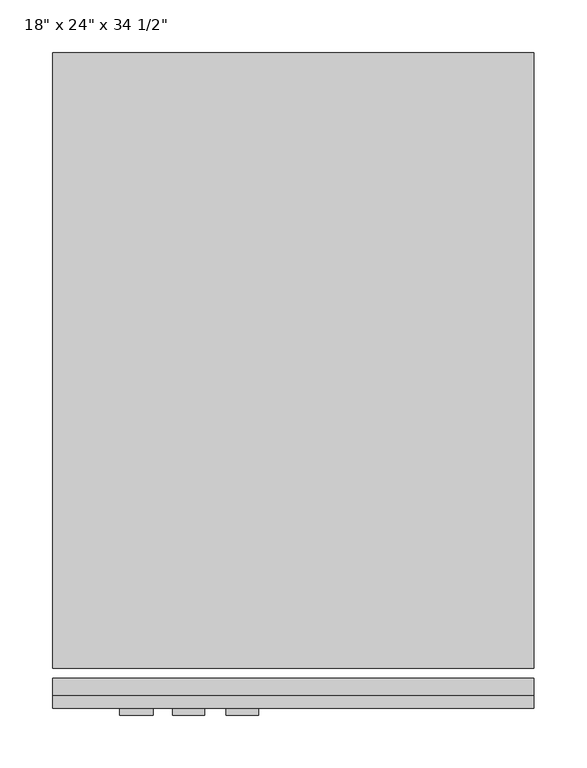
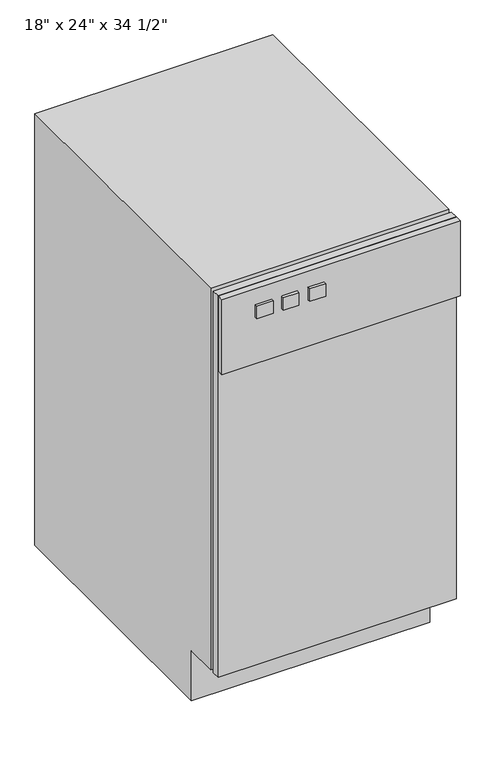
"""IFC4 building model written with IfcOpenShell, lengths in millimetres: proxy geometry."""

from ifc_helpers import new_model, si_unit, frame, origin, place, context, project, spatial, polyline, outline, extrude, source, transform, mapped, element, save


def proxy_7e1014cc(model_context):
    return source(origin(), model_context, "Body", "SweptSolid", [
        extrude(outline(polyline([(534.7174685, -38.3504352), (77.5174685, -38.3504352), (77.5174685, -22.4754352), (534.7174685, -22.4754352), (534.7174685, -38.3504352)])), frame((0.0, 0.0, 101.6), z_axis=(0.0, 0.0, 1.0), x_axis=(1.0, 0.0, 0.0)), (0.0, 0.0, 1.0), 774.7),
        extrude(outline(polyline([(534.7174685, -38.3504352), (534.7174685, -51.0504352), (77.5174685, -51.0504352), (77.5174685, -38.3504352), (534.7174685, -38.3504352)])), frame((0.0, 0.0, 723.9), z_axis=(0.0, 0.0, 1.0), x_axis=(1.0, 0.0, 0.0)), (0.0, 0.0, 1.0), 152.4),
        extrude(outline(polyline([(571.2495648, 0.0), (50.5495648, 0.0), (50.5495648, 101.6), (-12.9504352, 101.6), (-12.9504352, 876.3), (571.2495648, 876.3), (571.2495648, 0.0)])), frame((77.5174685, 0.0, 0.0), z_axis=(1.0, 0.0, 0.0), x_axis=(0.0, 1.0, 0.0)), (0.0, 0.0, 1.0), 457.2),
        extrude(outline(polyline([(172.7674685, -57.4004352), (141.0174685, -57.4004352), (141.0174685, -51.0504352), (172.7674685, -51.0504352), (172.7674685, -57.4004352)])), frame((0.0, 0.0, 818.6415009), z_axis=(0.0, 0.0, 1.0), x_axis=(1.0, 0.0, 0.0)), (0.0, 0.0, 1.0), 25.4),
        extrude(outline(polyline([(221.6847918, -57.4004352), (191.3389562, -57.4004352), (191.3389562, -51.0504352), (221.6847918, -51.0504352), (221.6847918, -57.4004352)])), frame((0.0, 0.0, 818.6415009), z_axis=(0.0, 0.0, 1.0), x_axis=(1.0, 0.0, 0.0)), (0.0, 0.0, 1.0), 25.4),
        extrude(outline(polyline([(272.969254, -57.4004352), (242.3199601, -57.4004352), (242.3199601, -51.0504352), (272.969254, -51.0504352), (272.969254, -57.4004352)])), frame((0.0, 0.0, 818.6415009), z_axis=(0.0, 0.0, 1.0), x_axis=(1.0, 0.0, 0.0)), (0.0, 0.0, 1.0), 25.4),
    ])


if __name__ == "__main__":
    model = new_model("IFC4")
    model_context = context("Model", 3, world=origin())
    ifc_project = project(units=[si_unit("LENGTHUNIT", "METRE", prefix="MILLI")], contexts=[model_context])
    site = spatial("IfcSite", under=ifc_project)
    building = spatial("IfcBuilding", under=site)
    placement = place(None, origin())
    proxy_shape = proxy_7e1014cc(model_context)
    element("IfcBuildingElementProxy", 1, Name="18\" x 24\" x 34 1/2\"", ObjectType="18\" x 24\" x 34 1/2\"", at=placement, inside=building, context=model_context, shape_type="MappedRepresentation", body=[
        mapped(proxy_shape, transform((0.0, 0.0, 0.0), x_axis=(1.0, 0.0, 0.0), y_axis=(0.0, 1.0, 0.0), z_axis=(0.0, 0.0, 1.0))),
    ])
    save(model, "model.ifc")

# Revit data of these elements
# Type "18\" x 24\" x 34 1/2\""
#   Label = "T"
#   Assembly Code = "E1090400"
#   Depth = 2' - 0"
#   Height = 2' - 10 1/2"
#   Width = 1' - 6"
#   Panel Face Material = Plastic, Opaque Black
#   Trach Compact. Material = Steel, Paint Finish, Ivory, Matte
#   Default Elevation = 0
# Element 1 (IfcBuildingElementProxy, "18\" x 24\" x 34 1/2\"")
#   Materials on its faces: "Steel, Paint Finish, Ivory, Matte", "Plastic, Opaque Black"
# Materials
#   "Plastic, Opaque Black": class "Plastic", colour RGB 0 0 0, transparency 0, Description = "Plastic, generic, opaque black", Cost = 0
#   "Steel, Paint Finish, Ivory, Matte": class "Metal", colour RGB 247 247 239, transparency 0, Description = "Steel, paint finish, ivory, matte", Cost = 0
